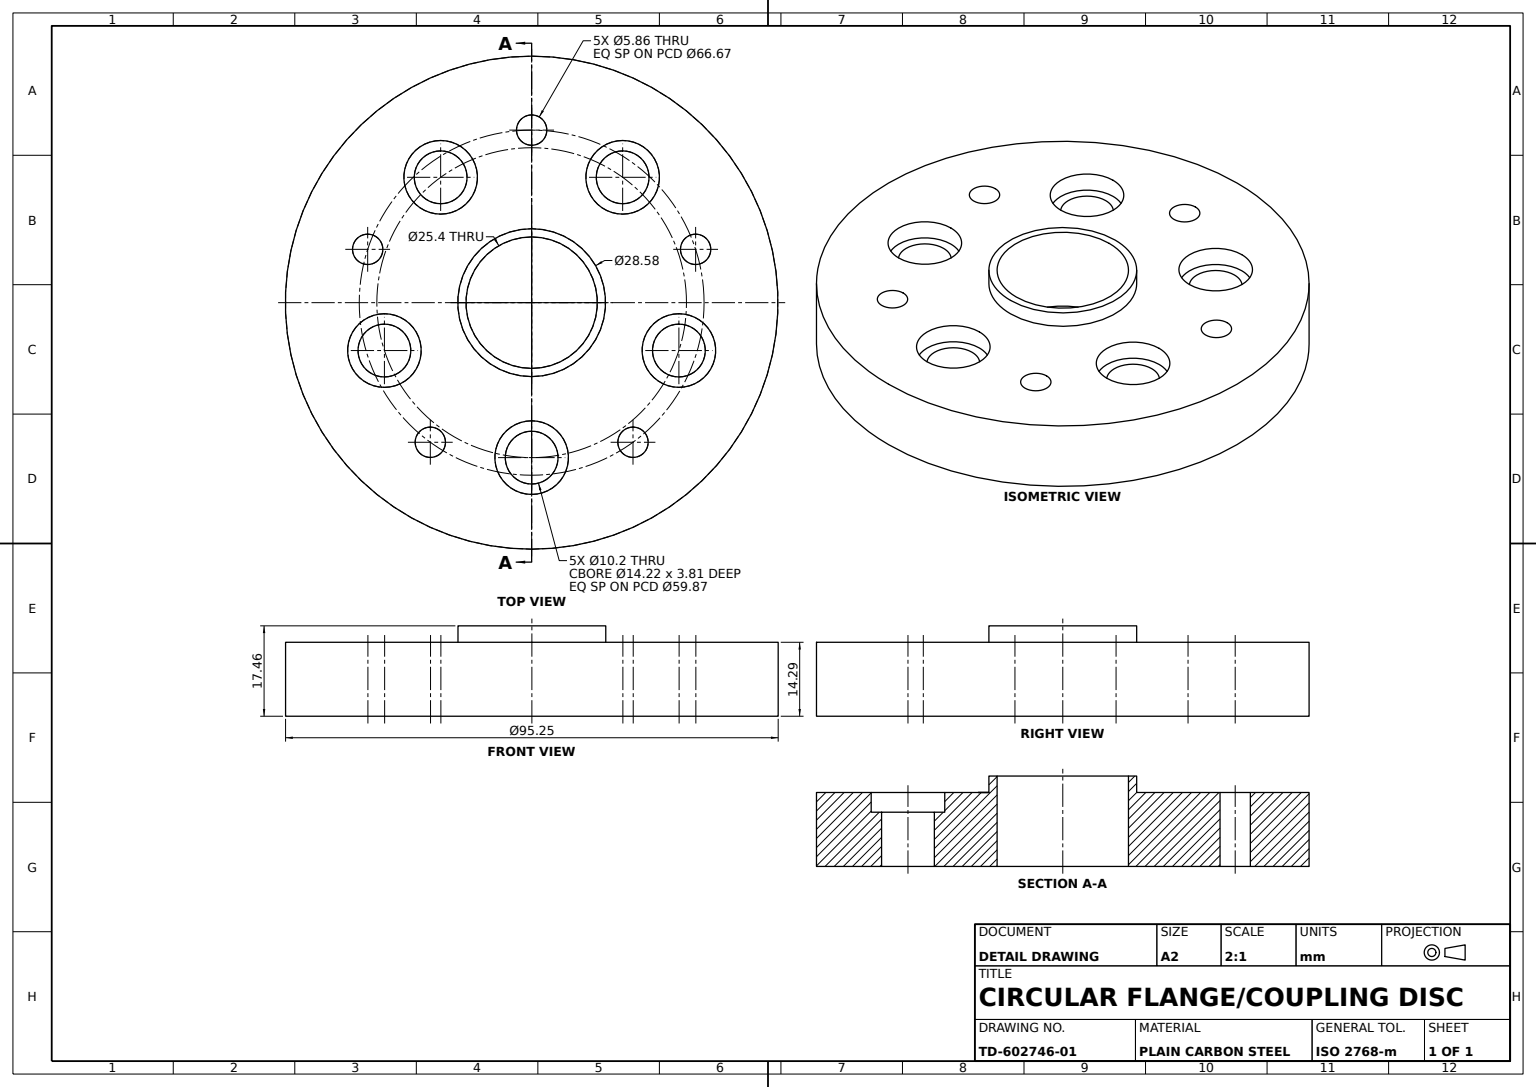
SolidWorks part; units mm, degrees
material "Plain Carbon Steel"
ref_plane "Front Plane" through (0, 0, 0) normal (0, 0, 1) x (1, 0, 0)
ref_plane "Top Plane" through (0, 0, 0) normal (0, 1, 0) x (1, 0, 0)
ref_plane "Right Plane" through (0, 0, 0) normal (1, 0, 0) x (0, 0, -1)
sketch "Flange Disc Sketch" plane through (0, 0, 0) normal (0, 1, 0) x (1, 0, 0)
  circle A0 centre (0, 0) radius 47.625
  dimension "D1" = 95.25
extrude "Flange Disc Ø3.75" add sketch "Flange Disc Sketch" along normal blind 14.2875
sketch "Tapped Holes Sketch" plane through (0, 14.2875, 0) normal (0, 1, 0) x (1, 0, 0)
  circle A0 centre (0, 0) radius 33.3375 construction
  circle A1 centre (0, 33.3375) radius 2.9307
  circle A2 centre (31.7058, 10.3019) radius 2.9307
  circle A3 centre (19.5953, -26.9706) radius 2.9307
  circle A4 centre (-19.5953, -26.9706) radius 2.9307
  circle A5 centre (-31.7058, 10.3019) radius 2.9307
  point P19 (0, 0)
  dimension "D1" = 66.675
  dimension "D2" = 5
  dimension "D3" = 5.8614
extrude "Tapped Holes 5x on BC Ø2.625" cut sketch "Tapped Holes Sketch" against normal blind 14.2875
sketch "Hub Boss Sketch" plane through (0, 14.2875, 0) normal (0, 1, 0) x (1, 0, 0)
  circle A0 centre (0, 0) radius 14.2875
  dimension "D1" = 28.575
extrude "Hub Boss Ø1.125" add sketch "Hub Boss Sketch" along normal blind 3.175
sketch "Center Bore Sketch" plane through (0, 17.4625, 0) normal (0, 1, 0) x (1, 0, 0)
  circle A0 centre (0, 0) radius 12.7
  dimension "D1" = 25.4
extrude "Center Bore Ø1.0" cut sketch "Center Bore Sketch" against normal blind 34.925
sketch "Counterbores Sketch" plane through (0, 14.2875, 0) normal (0, 1, 0) x (1, 0, 0)
  circle A0 centre (0, -29.9357) radius 7.112
  circle A1 centre (-28.4705, -9.2506) radius 7.112
  circle A2 centre (-17.5958, 24.2185) radius 7.112
  circle A3 centre (17.5958, 24.2185) radius 7.112
  circle A4 centre (28.4705, -9.2506) radius 7.112
  circle A5 centre (0, 33.3375) radius 2.9307 construction
  point P12 (0, 0)
  dimension "D1" = 14.224
  dimension "D3" = 17.5958
  dimension "D4" = 28.4705
  dimension "D5" = 9.119
  dimension "D2" = 5
extrude "Counterbores 5xØ0.56" cut sketch "Counterbores Sketch" against normal blind 3.81
sketch "Bolt Holes Sketch" plane through (0, 10.4775, 0) normal (0, 1, 0) x (1, 0, 0)
  circle A0 centre (0, -29.9357) radius 5.102
  circle A1 centre (-28.4705, -9.2506) radius 5.102
  circle A2 centre (-17.5958, 24.2185) radius 5.102
  circle A3 centre (17.5958, 24.2185) radius 5.102
  circle A4 centre (28.4705, -9.2506) radius 5.102
  circle A5 centre (0, -29.9357) radius 7.112 construction
  point P13 (0, 0)
  dimension "D2" = 10.204
  dimension "D3" = 17.5958
  dimension "D1" = 5
extrude "Counterbored Bolt Holes 5x" cut sketch "Bolt Holes Sketch" against normal blind 16.51
